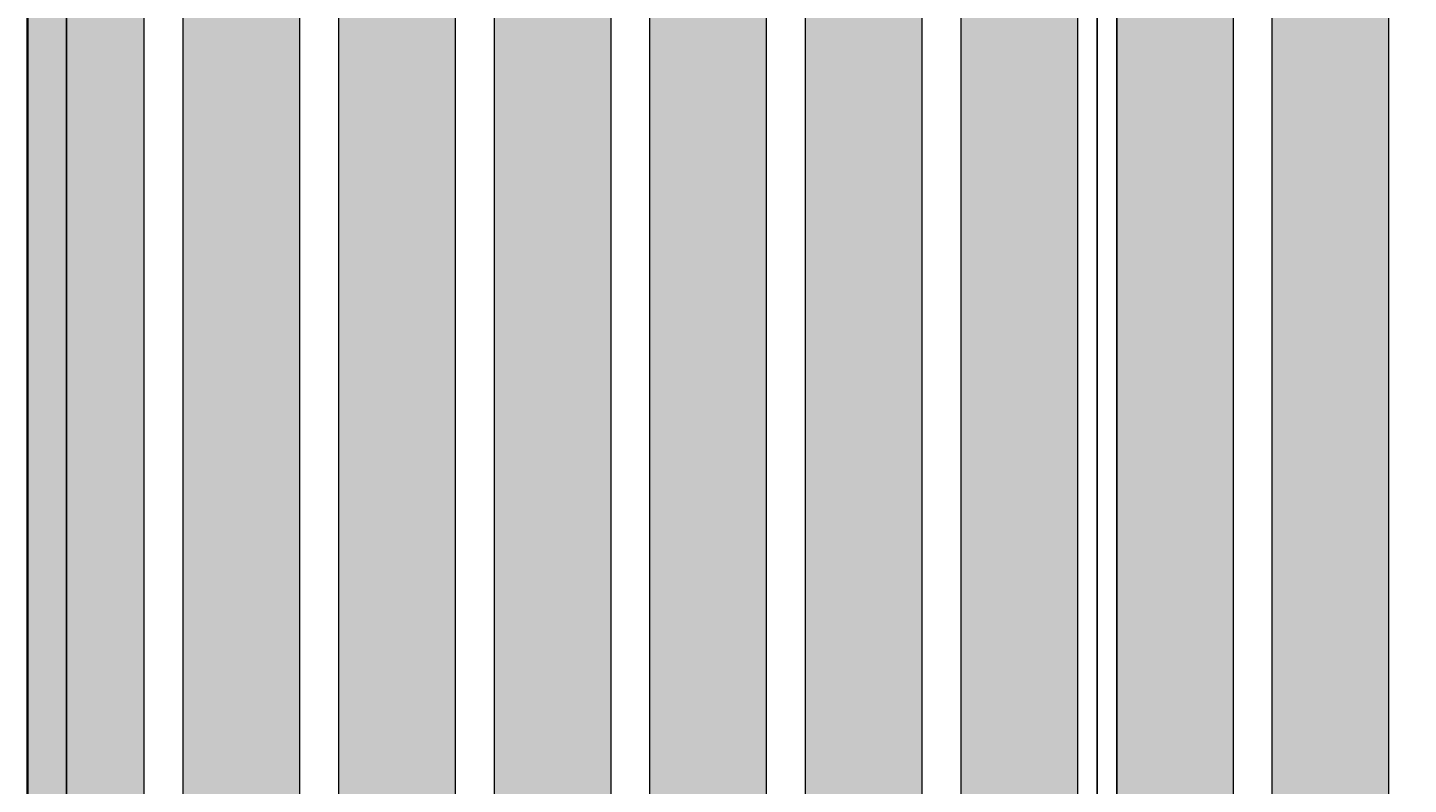
# Model space of a CAD drawing. Units: inches. Extents: x 4508 to 4723, y 847 to 1020.
# Tile 14 of 32: x 4550 to 4585, y 956 to 976. Entities that reach past the tile are written whole.
import ezdxf

# ---------------------------------------------------------------- set-up
doc = ezdxf.new("R2010")
doc.units = ezdxf.units.IN
for name, color, linetype, lineweight in [('A-ANNO-DIMS', 2, 'Continuous', 18), ('A-WALL', 7, 'Continuous', 35), ('A-WALL-FINS', 30, 'Continuous', 18), ('A-WALL-PATT', 254, 'Continuous', 13)]:
    doc.layers.add(name, color=color, linetype=linetype, lineweight=lineweight)
doc.styles.get("Standard").update_dxf_attribs({"font": 'arial.ttf'})
doc.dimstyles.get("Standard").update_dxf_attribs({"dimtxt": 0.18, "dimasz": 0.18, "dimexe": 0.18, "dimexo": 0.0625, "dimgap": 0.09, "dimtad": 0, "dimtih": 1, "dimtoh": 1, "dimdec": 4, "dimzin": 0, "dimdsep": 46, "dimtxsty": 'Standard', "dimcen": 0.09, "dimadec": 0, "dimazin": 0, "dimtfac": 1, "dimtdec": 4, "dimtofl": 0, "dimtmove": 0, "dimatfit": 3, "dimfxl": 1, "dimtolj": 1, "dimtzin": 0, "dimarcsym": 0})

# ---------------------------------------------------------------- blocks, each defined once
blk = doc.blocks.new('*D26')
at = {"layer": 'A-ANNO-DIMS', "color": 0, "lineweight": -2, "transparency": 16777216}
for p, q in [((4549.994, 904.809), (4549.994, 1002.877)), ((4550.994, 903.809), (4550.994, 1002.877)), ((4550.174, 1002.697), (4550.371, 1002.697)), ((4550.814, 1002.697), (4550.617, 1002.697))]:
    blk.add_line(p, q, dxfattribs=at)
at = {"layer": 'A-ANNO-DIMS', "color": 0, "lineweight": 9, "transparency": 16777216}
for points in [[(4550.174, 1002.727), (4550.174, 1002.667), (4549.994, 1002.697)], [(4550.814, 1002.727), (4550.814, 1002.667), (4550.994, 1002.697)]]:
    blk.add_solid(points, dxfattribs=at)
at = {"layer": 'Defpoints', "color": 0, "lineweight": 9, "transparency": 16777216}
for p in [(4550.994, 1002.697), (4549.994, 904.747), (4550.994, 903.747)]:
    blk.add_point(p, dxfattribs=at)
at = {"layer": 'A-ANNO-DIMS', "color": 0, "transparency": 16777216, "insert": (4550.494, 1002.697), "char_height": 0.18, "attachment_point": 5}
blk.add_mtext('\\A1;1', dxfattribs=at)
blk = doc.blocks.new('*D27')
at = {"layer": 'A-ANNO-DIMS', "color": 0, "lineweight": -2, "transparency": 16777216}
for p, q in [((4550.994, 903.809), (4550.994, 1002.877)), ((4577.494, 903.809), (4577.494, 1002.877)), ((4551.174, 1002.697), (4563.918, 1002.697)), ((4577.314, 1002.697), (4564.57, 1002.697))]:
    blk.add_line(p, q, dxfattribs=at)
at = {"layer": 'A-ANNO-DIMS', "color": 0, "lineweight": 9, "transparency": 16777216}
for points in [[(4551.174, 1002.727), (4551.174, 1002.667), (4550.994, 1002.697)], [(4577.314, 1002.727), (4577.314, 1002.667), (4577.494, 1002.697)]]:
    blk.add_solid(points, dxfattribs=at)
at = {"layer": 'Defpoints', "color": 0, "lineweight": 9, "transparency": 16777216}
for p in [(4577.494, 1002.697), (4550.994, 903.747), (4577.494, 903.747)]:
    blk.add_point(p, dxfattribs=at)
at = {"layer": 'A-ANNO-DIMS', "color": 0, "transparency": 16777216, "insert": (4564.244, 1002.697), "char_height": 0.18, "attachment_point": 5}
blk.add_mtext('\\A1;26.5', dxfattribs=at)
blk = doc.blocks.new('*D28')
at = {"layer": 'A-ANNO-DIMS', "color": 0, "lineweight": -2, "transparency": 16777216}
for p, q in [((4577.494, 903.809), (4577.494, 1002.877)), ((4577.994, 903.809), (4577.994, 1002.877)), ((4577.314, 1002.697), (4577.134, 1002.697)), ((4578.174, 1002.697), (4578.354, 1002.697))]:
    blk.add_line(p, q, dxfattribs=at)
at = {"layer": 'A-ANNO-DIMS', "color": 0, "lineweight": 9, "transparency": 16777216}
for points in [[(4577.314, 1002.727), (4577.314, 1002.667), (4577.494, 1002.697)], [(4578.174, 1002.727), (4578.174, 1002.667), (4577.994, 1002.697)]]:
    blk.add_solid(points, dxfattribs=at)
at = {"layer": 'Defpoints', "color": 0, "lineweight": 9, "transparency": 16777216}
for p in [(4577.994, 1002.697), (4577.494, 903.747), (4577.994, 903.747)]:
    blk.add_point(p, dxfattribs=at)
at = {"layer": 'A-ANNO-DIMS', "color": 0, "transparency": 16777216, "insert": (4578.608, 1002.697), "char_height": 0.18, "attachment_point": 5}
blk.add_mtext('\\A1;0.5', dxfattribs=at)
blk = doc.blocks.new('*D29')
at = {"layer": 'A-ANNO-DIMS', "color": 0, "lineweight": -2, "transparency": 16777216}
for p, q in [((4577.994, 903.809), (4577.994, 1002.877)), ((4603.994, 903.809), (4603.994, 1002.877)), ((4578.174, 1002.697), (4590.773, 1002.697)), ((4603.814, 1002.697), (4591.214, 1002.697))]:
    blk.add_line(p, q, dxfattribs=at)
at = {"layer": 'A-ANNO-DIMS', "color": 0, "lineweight": 9, "transparency": 16777216}
for points in [[(4578.174, 1002.727), (4578.174, 1002.667), (4577.994, 1002.697)], [(4603.814, 1002.727), (4603.814, 1002.667), (4603.994, 1002.697)]]:
    blk.add_solid(points, dxfattribs=at)
at = {"layer": 'Defpoints', "color": 0, "lineweight": 9, "transparency": 16777216}
for p in [(4603.994, 1002.697), (4577.994, 903.747), (4603.994, 903.747)]:
    blk.add_point(p, dxfattribs=at)
at = {"layer": 'A-ANNO-DIMS', "color": 0, "transparency": 16777216, "insert": (4590.994, 1002.697), "char_height": 0.18, "attachment_point": 5}
blk.add_mtext('\\A1;26', dxfattribs=at)

msp = doc.modelspace()

# ---------------------------------------------------------------- hatches: boundary and pattern name
at = {"layer": 'A-WALL-PATT', "transparency": 33554681}
h = msp.add_hatch(color=256, dxfattribs=at)
h.dxf.hatch_style = 1
h.paths.add_polyline_path([(4552.9938, 994.7469), (4549.9938, 994.7469), (4549.9938, 904.7469), (4552.9938, 904.7469)])
h.paths.add_polyline_path([(4556.9938, 994.7469), (4553.9938, 994.7469), (4553.9938, 904.7469), (4556.9938, 904.7469)])
h.paths.add_polyline_path([(4560.9938, 994.7469), (4557.9938, 994.7469), (4557.9938, 904.7469), (4560.9938, 904.7469)])
h.paths.add_polyline_path([(4564.9938, 994.7469), (4561.9938, 994.7469), (4561.9938, 904.7469), (4564.9938, 904.7469)])
h.paths.add_polyline_path([(4568.9938, 994.7469), (4565.9938, 994.7469), (4565.9938, 904.7469), (4568.9938, 904.7469)])
h.paths.add_polyline_path([(4572.9938, 994.7469), (4569.9938, 994.7469), (4569.9938, 904.7469), (4572.9938, 904.7469)])
h.paths.add_polyline_path([(4576.9938, 994.7469), (4573.9938, 994.7469), (4573.9938, 904.7469), (4576.9938, 904.7469)])
h.paths.add_polyline_path([(4580.9938, 994.7469), (4577.9938, 994.7469), (4577.9938, 904.7469), (4580.9938, 904.7469)])
h.paths.add_polyline_path([(4584.9938, 994.7469), (4581.9938, 994.7469), (4581.9938, 904.7469), (4584.9938, 904.7469)])

# ---------------------------------------------------------------- linework, layer by layer
at = {"layer": 'A-WALL'}
msp.add_line((4549.9938, 874.7469), (4549.9938, 994.7469), dxfattribs=at)
at = {"layer": 'A-WALL-FINS'}
for p, q in [((4552.9938, 904.7469), (4552.9938, 994.7469)), ((4553.9938, 904.7469), (4553.9938, 994.7469)), ((4556.9938, 904.7469), (4556.9938, 994.7469)), ((4557.9938, 904.7469), (4557.9938, 994.7469)), ((4560.9938, 904.7469), (4560.9938, 994.7469)), ((4561.9938, 904.7469), (4561.9938, 994.7469)), ((4564.9938, 904.7469), (4564.9938, 994.7469)), ((4565.9938, 904.7469), (4565.9938, 994.7469)), ((4568.9938, 904.7469), (4568.9938, 994.7469)), ((4569.9938, 904.7469), (4569.9938, 994.7469)), ((4572.9938, 904.7469), (4572.9938, 994.7469)), ((4573.9938, 904.7469), (4573.9938, 994.7469)), ((4576.9938, 904.7469), (4576.9938, 994.7469)), ((4577.9938, 904.7469), (4577.9938, 994.7469)), ((4580.9938, 904.7469), (4580.9938, 994.7469)), ((4581.9938, 904.7469), (4581.9938, 994.7469)), ((4584.9938, 904.7469), (4584.9938, 994.7469))]:
    msp.add_line(p, q, dxfattribs=at)

# ---------------------------------------------------------------- dimensions: what is measured, and where the dimension line sits
at = {"layer": 'A-ANNO-DIMS'}
for base, p1, p2, override, picture, middle in [((4550.9938, 1002.6969), (4549.9938, 904.7469), (4550.9938, 903.7469), {"dimdec": 0, "dimlfac": 1, "dimrnd": 0, "dimzin": 0, "dimdsep": 46, "dimlunit": 2}, '*D26', (4550.4938, 1002.6969)), ((4577.4938, 1002.6969), (4550.9938, 903.7469), (4577.4938, 903.7469), {"dimdec": 1, "dimlfac": 1, "dimrnd": 0, "dimzin": 0, "dimdsep": 46, "dimlunit": 2}, '*D27', (4564.2438, 1002.6969)), ((4577.9938, 1002.6969), (4577.4938, 903.7469), (4577.9938, 903.7469), {"dimdec": 1, "dimlfac": 1, "dimrnd": 0, "dimzin": 0, "dimdsep": 46, "dimlunit": 2}, '*D28', (4578.6083, 1002.6969)), ((4603.9938, 1002.6969), (4577.9938, 903.7469), (4603.9938, 903.7469), {"dimdec": 0, "dimlfac": 1, "dimrnd": 0, "dimzin": 0, "dimdsep": 46, "dimlunit": 2}, '*D29', (4590.9938, 1002.6969))]:
    dim = msp.add_linear_dim(base=base, p1=p1, p2=p2, dimstyle='Standard', override=override, dxfattribs=at)
    dim.commit()
    dim.dimension.update_dxf_attribs({"geometry": picture, "text_midpoint": middle})

doc.saveas('drawing.dxf')
